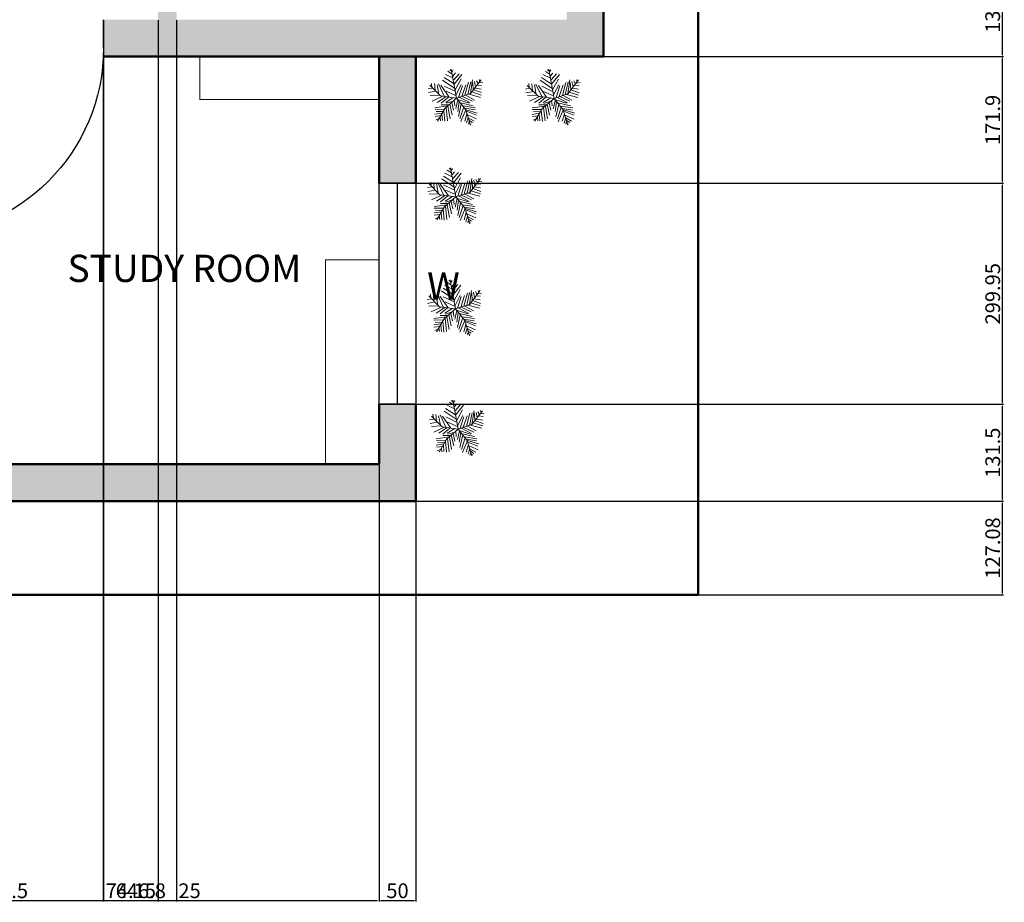
# Model space of a CAD drawing. Units: millimetres. Extents: x 1898 to 8115, y 727 to 4291.
# Tile 6 of 7: x 6778 to 8115, y 1079 to 2277. Entities that reach past the tile are written whole.
import ezdxf

# ---------------------------------------------------------------- set-up
doc = ezdxf.new("R2010")
doc.units = ezdxf.units.MM
for name, color, linetype, lineweight in [('A-ANNO-DIMS', 2, 'Continuous', 18), ('A-ANNO-TEXT', 7, 'Continuous', 25), ('A-AREA-IDEN', 3, 'Continuous', 25), ('A-DOOR', 3, 'Continuous', 25), ('A-FURN', 8, 'Continuous', 18), ('A-GLAZ', 4, 'Continuous', 25), ('A-WALL', 7, 'Continuous', 50), ('A-WALL-PATT', 8, 'Continuous', 13), ('L-PLNT', 112, 'Continuous', 18)]:
    doc.layers.add(name, color=color, linetype=linetype, lineweight=lineweight)
doc.styles.get("Standard").update_dxf_attribs({"font": 'arial.ttf'})
doc.dimstyles.new('ISO-25', dxfattribs={"dimtxt": 20, "dimasz": 2.5, "dimexe": 1.25, "dimexo": 0.625, "dimtad": 1, "dimtxsty": 'Standard', "dimcen": 2.5, "dimadec": 0, "dimazin": 0, "dimtfac": 1, "dimtmove": 0, "dimatfit": 3, "dimfxl": 1, "dimarcsym": 0})

# ---------------------------------------------------------------- blocks, each defined once
blk = doc.blocks.new('*U43')
for p, q in [((0, 0), (0, -6)), ((40, 0), (40, -6))]:
    blk.add_line(p, q)
blk.add_lwpolyline([(0, 0), (0, 40), (1.75, 40), (1.75, 0)], close=True)
blk.add_arc((0, 0), 40, 0, 90)
blk = doc.blocks.new('*U47')
for p, q in [((-5.114, 28.097), (-24.676, 40.636)), ((-7.288, 39.707), (-21.778, 46.673)), ((-8.737, 47.138), (-17.069, 52.711)), ((-10.186, 53.64), (-13.084, 55.962)), ((0, 0), (-10.5, 57)), ((-9.099, 51.782), (-6.563, 55.962)), ((-7.65, 43.423), (-2.578, 49.46)), ((-5.839, 35.992), (4.667, 48.067)), ((-5.114, 27.632), (10.463, 46.673)), ((-47.498, 19.737), (-55.83, 18.344)), ((-31.5, 4.5), (-52.5, 25.5)), ((-48.585, 21.131), (-49.309, 29.026)), ((-43.513, 28.561), (-42.427, 15.558)), ((-38.442, 26.239), (-34.819, 7.663)), ((-35.544, 28.097), (-24.314, 3.947)), ((-14.533, 2.09), (-30.834, 25.31)), ((-3.665, 19.273), (-27.574, 35.527)), ((-24.314, 23.917), (-2.941, 13.7)), ((-2.941, 16.486), (8.652, 37.85)), ((-1.129, 6.734), (9.014, 26.704)), ((3.942, 1.625), (11.187, 24.381)), ((10.101, 3.483), (17.708, 26.239)), ((16.259, 5.805), (23.142, 31.348)), ((22.055, 7.198), (27.489, 32.277)), ((27, 9), (48, 36)), ((27.127, 9.056), (31.112, 35.992)), ((31.836, 30.883), (32.561, 16.486)), ((35.096, 32.741), (37.27, 22.524)), ((36.183, 19.737), (48.137, 17.88)), ((38.719, 34.134), (41.979, 28.561)), ((40.53, 25.775), (48.862, 24.846)), ((43.791, 29.954), (51.036, 30.883)), ((44.153, 36.456), (45.239, 32.741)), ((-40.615, 13.7), (-55.105, 10.913)), ((-33.37, 6.269), (-52.207, 5.34)), ((-28.299, 3.483), (-47.86, -5.805)), ((-21.416, 3.018), (-38.079, -8.128)), ((0, 0), (-31.5, 4.5)), ((-15.982, 2.09), (-30.11, -9.521)), ((0, 0), (-22.5, -19.5)), ((-6.563, 1.161), (-21.416, -8.128)), ((-20.691, 13.7), (-1.129, 4.876)), ((0, 0), (27, 9)), ((0, 0), (18, -22.5)), ((6.478, 1.625), (26.04, -8.592)), ((11.187, 3.483), (30.749, -5.805)), ((18.07, 5.805), (35.096, -3.483)), ((24.229, 7.663), (46.688, 1.625)), ((29.662, 12.307), (48.137, 6.269)), ((33.285, 16.486), (48.862, 10.913)), ((-17.431, -15.094), (-42.789, -18.809)), ((-15.257, -12.772), (-30.11, -12.772)), ((-20.691, -18.345), (-17.793, -44.352)), ((-6.563, -5.805), (-19.967, -9.985)), ((-17.069, -15.094), (-12.721, -40.172)), ((-13.446, -11.378), (-8.737, -32.741)), ((-9.461, -8.592), (-6.201, -23.453)), ((-4.752, -3.483), (-3.665, -14.629)), ((2.493, -3.019), (-1.491, -20.202)), ((1.769, -2.555), (24.229, -9.521)), ((5.029, -6.27), (2.131, -25.775)), ((9.014, -11.378), (3.58, -35.992)), ((14.085, -16.951), (6.478, -40.172)), ((7.565, -9.056), (32.198, -14.629)), ((12.274, -15.094), (36.907, -18.809)), ((-28.299, -29.026), (-42.789, -31.348)), ((-24.314, -21.596), (-42.427, -22.06)), ((-30.834, -34.135), (-42.427, -35.528)), ((-26.849, -26.24), (-40.253, -25.775)), ((-22.5, -19.5), (-37.5, -45)), ((-32.646, -36.921), (-31.921, -44.352)), ((-29.023, -30.884), (-27.936, -43.887)), ((-25.038, -23.918), (-22.865, -45.281)), ((18.07, -22.524), (8.289, -45.745)), ((20.244, -30.419), (15.897, -44.816)), ((16.259, -19.738), (36.183, -22.989)), ((18, -22.5), (27, -52.5)), ((18.433, -22.524), (40.53, -29.026)), ((19.157, -25.311), (38.719, -33.206)), ((22.78, -37.85), (19.519, -48.532)), ((21.331, -32.741), (39.081, -40.636)), ((22.78, -38.314), (34.372, -44.816)), ((-34.457, -39.708), (-40.978, -42.494)), ((24.591, -45.745), (23.142, -50.854)), ((24.591, -43.423), (30.749, -47.603)), ((26.764, -49.925), (28.213, -50.854))]:
    blk.add_line(p, q)
blk = doc.blocks.new('*D62')
at = {"layer": 'A-ANNO-DIMS', "color": 0, "lineweight": -2, "transparency": 16777216}
for p, q in [((7316.4, 1623.6), (8113.5, 1623.6)), ((8112.2, 1499), (8112.2, 1621.1)), ((7699.4, 1496.5), (8113.5, 1496.5))]:
    blk.add_line(p, q, dxfattribs=at)
at = {"layer": 'A-ANNO-DIMS', "color": 0, "transparency": 16777216}
for points in [[(8111.8, 1621.1), (8112.7, 1621.1), (8112.2, 1623.6)], [(8111.8, 1499), (8112.7, 1499), (8112.2, 1496.5)]]:
    blk.add_solid(points, dxfattribs=at)
at = {"layer": 'Defpoints', "color": 0, "transparency": 16777216}
for p in [(7315.8, 1623.6), (8112.2, 1623.6), (7698.8, 1496.5)]:
    blk.add_point(p, dxfattribs=at)
at = {"layer": 'A-ANNO-DIMS', "color": 0, "transparency": 16777216, "insert": (8101.4, 1560.1), "char_height": 20, "attachment_point": 5, "rotation": 90}
blk.add_mtext('127.08', dxfattribs=at)
blk = doc.blocks.new('*D77')
at = {"layer": 'A-ANNO-DIMS', "color": 0, "lineweight": -2, "transparency": 16777216}
for p, q in [((6618.9, 1673), (6618.9, 1080.3)), ((7265.8, 1673), (7265.8, 1080.3)), ((6621.4, 1081.6), (7263.3, 1081.6))]:
    blk.add_line(p, q, dxfattribs=at)
at = {"layer": 'A-ANNO-DIMS', "color": 0, "transparency": 16777216}
for points in [[(6621.4, 1082), (6621.4, 1081.2), (6618.9, 1081.6)], [(7263.3, 1082), (7263.3, 1081.2), (7265.8, 1081.6)]]:
    blk.add_solid(points, dxfattribs=at)
at = {"layer": 'Defpoints', "color": 0, "transparency": 16777216}
for p in [(6618.9, 1673.6), (7265.8, 1673.6), (7265.8, 1081.6)]:
    blk.add_point(p, dxfattribs=at)
at = {"layer": 'A-ANNO-DIMS', "color": 0, "transparency": 16777216, "insert": (6942.3, 1092.4), "char_height": 20, "attachment_point": 5}
blk.add_mtext('646.8', dxfattribs=at)
blk = doc.blocks.new('*D78')
at = {"layer": 'A-ANNO-DIMS', "color": 0, "lineweight": -2, "transparency": 16777216}
for p, q in [((7265.8, 1673), (7265.8, 1080.3)), ((7315.8, 1623), (7315.8, 1080.3)), ((7268.3, 1081.6), (7313.3, 1081.6))]:
    blk.add_line(p, q, dxfattribs=at)
at = {"layer": 'A-ANNO-DIMS', "color": 0, "transparency": 16777216}
for points in [[(7268.3, 1082), (7268.3, 1081.2), (7265.8, 1081.6)], [(7313.3, 1082), (7313.3, 1081.2), (7315.8, 1081.6)]]:
    blk.add_solid(points, dxfattribs=at)
at = {"layer": 'Defpoints', "color": 0, "transparency": 16777216}
for p in [(7265.8, 1673.6), (7315.8, 1623.6), (7315.8, 1081.6)]:
    blk.add_point(p, dxfattribs=at)
at = {"layer": 'A-ANNO-DIMS', "color": 0, "transparency": 16777216, "insert": (7290.8, 1092.4), "char_height": 20, "attachment_point": 5}
blk.add_mtext('50', dxfattribs=at)
blk = doc.blocks.new('*D91')
at = {"layer": 'A-ANNO-DIMS', "color": 0, "lineweight": -2, "transparency": 16777216}
for p, q in [((7316.4, 1755.1), (8113.5, 1755.1)), ((8112.2, 1626.1), (8112.2, 1752.6)), ((7316.4, 1623.6), (8113.5, 1623.6))]:
    blk.add_line(p, q, dxfattribs=at)
at = {"layer": 'A-ANNO-DIMS', "color": 0, "transparency": 16777216}
for points in [[(8111.8, 1752.6), (8112.7, 1752.6), (8112.2, 1755.1)], [(8111.8, 1626.1), (8112.7, 1626.1), (8112.2, 1623.6)]]:
    blk.add_solid(points, dxfattribs=at)
at = {"layer": 'Defpoints', "color": 0, "transparency": 16777216}
for p in [(7315.8, 1755.1), (8112.2, 1755.1), (7315.8, 1623.6)]:
    blk.add_point(p, dxfattribs=at)
at = {"layer": 'A-ANNO-DIMS', "color": 0, "transparency": 16777216, "insert": (8101.4, 1689.4), "char_height": 20, "attachment_point": 5, "rotation": 90}
blk.add_mtext('131.5', dxfattribs=at)
blk = doc.blocks.new('*D92')
at = {"layer": 'A-ANNO-DIMS', "color": 0, "lineweight": -2, "transparency": 16777216}
for p, q in [((7316.4, 2055.1), (8113.5, 2055.1)), ((8112.2, 1757.6), (8112.2, 2052.6)), ((7316.4, 1755.1), (8113.5, 1755.1))]:
    blk.add_line(p, q, dxfattribs=at)
at = {"layer": 'A-ANNO-DIMS', "color": 0, "transparency": 16777216}
for points in [[(8111.8, 2052.6), (8112.7, 2052.6), (8112.2, 2055.1)], [(8111.8, 1757.6), (8112.7, 1757.6), (8112.2, 1755.1)]]:
    blk.add_solid(points, dxfattribs=at)
at = {"layer": 'Defpoints', "color": 0, "transparency": 16777216}
for p in [(7315.8, 2055.1), (8112.2, 2055.1), (7315.8, 1755.1)]:
    blk.add_point(p, dxfattribs=at)
at = {"layer": 'A-ANNO-DIMS', "color": 0, "transparency": 16777216, "insert": (8101.4, 1905.1), "char_height": 20, "attachment_point": 5, "rotation": 90}
blk.add_mtext('299.95', dxfattribs=at)
blk = doc.blocks.new('*D93')
at = {"layer": 'A-ANNO-DIMS', "color": 0, "lineweight": -2, "transparency": 16777216}
for p, q in [((7316.4, 2227), (8113.5, 2227)), ((8112.2, 2057.6), (8112.2, 2224.5)), ((7316.4, 2055.1), (8113.5, 2055.1))]:
    blk.add_line(p, q, dxfattribs=at)
at = {"layer": 'A-ANNO-DIMS', "color": 0, "transparency": 16777216}
for points in [[(8111.8, 2224.5), (8112.7, 2224.5), (8112.2, 2227)], [(8111.8, 2057.6), (8112.7, 2057.6), (8112.2, 2055.1)]]:
    blk.add_solid(points, dxfattribs=at)
at = {"layer": 'Defpoints', "color": 0, "transparency": 16777216}
for p in [(7315.8, 2227), (8112.2, 2227), (7315.8, 2055.1)]:
    blk.add_point(p, dxfattribs=at)
at = {"layer": 'A-ANNO-DIMS', "color": 0, "transparency": 16777216, "insert": (8101.4, 2141), "char_height": 20, "attachment_point": 5, "rotation": 90}
blk.add_mtext('171.9', dxfattribs=at)
blk = doc.blocks.new('*D94')
at = {"layer": 'A-ANNO-DIMS', "color": 0, "lineweight": -2, "transparency": 16777216}
for p, q in [((7570.8, 2359.5), (8113.5, 2359.5)), ((8112.2, 2229.5), (8112.2, 2357)), ((7570.8, 2227), (8113.5, 2227))]:
    blk.add_line(p, q, dxfattribs=at)
at = {"layer": 'A-ANNO-DIMS', "color": 0, "transparency": 16777216}
for points in [[(8111.8, 2357), (8112.7, 2357), (8112.2, 2359.5)], [(8111.8, 2229.5), (8112.7, 2229.5), (8112.2, 2227)]]:
    blk.add_solid(points, dxfattribs=at)
at = {"layer": 'Defpoints', "color": 0, "transparency": 16777216}
for p in [(7570.2, 2359.5), (8112.2, 2359.5), (7570.2, 2227)]:
    blk.add_point(p, dxfattribs=at)
at = {"layer": 'A-ANNO-DIMS', "color": 0, "transparency": 16777216, "insert": (8101.4, 2293.2), "char_height": 20, "attachment_point": 5, "rotation": 90}
blk.add_mtext('132.5', dxfattribs=at)
blk = doc.blocks.new('*D107')
at = {"layer": 'A-ANNO-DIMS', "color": 0, "lineweight": -2, "transparency": 16777216}
for p, q in [((6618.9, 2226.3), (6618.9, 1080.3)), ((6891.4, 2226.3), (6891.4, 1080.3)), ((6621.4, 1081.6), (6888.9, 1081.6))]:
    blk.add_line(p, q, dxfattribs=at)
at = {"layer": 'A-ANNO-DIMS', "color": 0, "transparency": 16777216}
for points in [[(6621.4, 1082), (6621.4, 1081.2), (6618.9, 1081.6)], [(6888.9, 1082), (6888.9, 1081.2), (6891.4, 1081.6)]]:
    blk.add_solid(points, dxfattribs=at)
at = {"layer": 'Defpoints', "color": 0, "transparency": 16777216}
for p in [(6618.9, 2227), (6891.4, 2227), (6891.4, 1081.6)]:
    blk.add_point(p, dxfattribs=at)
at = {"layer": 'A-ANNO-DIMS', "color": 0, "transparency": 16777216, "insert": (6755.2, 1092.4), "char_height": 20, "attachment_point": 5}
blk.add_mtext('272.5', dxfattribs=at)
blk = doc.blocks.new('*D108')
at = {"layer": 'A-ANNO-DIMS', "color": 0, "lineweight": -2, "transparency": 16777216}
for p, q in [((6891.7, 2276.3), (6891.7, 1080.3)), ((6965.8, 2276.3), (6965.8, 1080.3)), ((6894.2, 1081.6), (6963.3, 1081.6))]:
    blk.add_line(p, q, dxfattribs=at)
at = {"layer": 'A-ANNO-DIMS', "color": 0, "transparency": 16777216}
for points in [[(6894.2, 1082), (6894.2, 1081.2), (6891.7, 1081.6)], [(6963.3, 1082), (6963.3, 1081.2), (6965.8, 1081.6)]]:
    blk.add_solid(points, dxfattribs=at)
at = {"layer": 'Defpoints', "color": 0, "transparency": 16777216}
for p in [(6891.7, 2277), (6965.8, 2277), (6965.8, 1081.6)]:
    blk.add_point(p, dxfattribs=at)
at = {"layer": 'A-ANNO-DIMS', "color": 0, "transparency": 16777216, "insert": (6928.8, 1092.4), "char_height": 20, "attachment_point": 5}
blk.add_mtext('74.15', dxfattribs=at)
blk = doc.blocks.new('*D109')
at = {"layer": 'A-ANNO-DIMS', "color": 0, "lineweight": -2, "transparency": 16777216}
for p, q in [((6965.8, 2276.3), (6965.8, 1080.3)), ((6990.8, 2276.3), (6990.8, 1080.3)), ((6968.3, 1081.6), (6988.3, 1081.6)), ((6990.8, 1081.6), (7023.7, 1081.6))]:
    blk.add_line(p, q, dxfattribs=at)
at = {"layer": 'A-ANNO-DIMS', "color": 0, "transparency": 16777216}
for points in [[(6968.3, 1082), (6968.3, 1081.2), (6965.8, 1081.6)], [(6988.3, 1082), (6988.3, 1081.2), (6990.8, 1081.6)]]:
    blk.add_solid(points, dxfattribs=at)
at = {"layer": 'Defpoints', "color": 0, "transparency": 16777216}
for p in [(6965.8, 2277), (6990.8, 2277), (6990.8, 1081.6)]:
    blk.add_point(p, dxfattribs=at)
at = {"layer": 'A-ANNO-DIMS', "color": 0, "transparency": 16777216, "insert": (7008.5, 1092.4), "char_height": 20, "attachment_point": 5}
blk.add_mtext('25', dxfattribs=at)

msp = doc.modelspace()

# ---------------------------------------------------------------- hatches: boundary and pattern name
at = {"layer": 'A-WALL-PATT'}
h = msp.add_hatch(color=256, dxfattribs=at)
h.dxf.hatch_style = 1
h.paths.add_polyline_path([(6201.726, 3440.661), (5461.585, 3440.661), (5461.585, 3265.221), (5511.585, 3265.221), (5511.585, 3390.661), (6176.726, 3390.661), (6176.726, 2856.284), (6201.726, 2856.284)])
h.paths.add_polyline_path([(6784.895, 3318.017), (6201.726, 3318.017), (6201.726, 3268.017), (6784.895, 3268.017)])
h.paths.add_polyline_path([(7570.217, 3440.661), (6784.895, 3440.661), (6784.895, 3057.009), (6809.895, 3057.009), (6809.895, 3390.661), (7520.217, 3390.661), (7520.217, 3300.311), (7570.217, 3300.311)])
h.paths.add_polyline_path([(7570.217, 3000.359), (7520.217, 3000.359), (7520.217, 2758.681), (7570.217, 2758.681)])
h.paths.add_polyline_path([(7520.217, 2856.284), (7194.283, 2856.284), (6784.895, 2856.284), (6784.895, 2831.284), (7520.217, 2831.284)])
h.paths.add_polyline_path([(6809.895, 2878.069), (6784.895, 2878.069), (6784.895, 2856.284), (6809.895, 2856.284)])
h.paths.add_polyline_path([(6201.726, 2856.284), (6176.726, 2856.284), (6161.551, 2856.284), (6161.551, 2831.284), (6201.726, 2831.284)])
h.paths.add_polyline_path([(5905.861, 2856.284), (5511.585, 2856.284), (5511.585, 2831.284), (5905.861, 2831.284)])
h.paths.add_polyline_path([(5511.585, 2965.269), (5461.585, 2965.269), (5461.585, 2698.678), (5511.585, 2698.678)])
h.paths.add_polyline_path([(5511.585, 2398.725), (5461.585, 2398.725), (5461.585, 2088.028), (5511.585, 2088.028)])
h.paths.add_polyline_path([(5989.6, 2238.621), (5989.6, 2276.975), (5511.585, 2276.975), (5511.585, 2226.975), (5989.865, 2226.975, -0.01139164)])
h.paths.add_polyline_path([(6636.013, 2276.975), (6245.29, 2276.975), (6245.29, 2238.621), (6245.29, 2226.975), (6636.013, 2226.975), (6636.013, 2238.621)])
h.paths.add_polyline_path([(7570.217, 2359.481), (7520.217, 2359.481), (7520.217, 2326.802), (7520.217, 2276.975), (6891.704, 2276.975), (6891.704, 2238.621, -0.01139164), (6891.439, 2226.975), (7570.217, 2226.975)])
h.paths.add_polyline_path([(7145.586, 2531.644), (6989.313, 2531.644), (6989.313, 2538.488), (7145.735, 2538.488), (7145.735, 2531.644), (7145.586, 2531.644, -0.39860379), (6990.849, 2382.073), (6990.849, 2276.975), (6965.849, 2276.975), (6965.849, 2382.065), (6989.313, 2382.065, 0.40145271)])
h.paths.add_polyline_path([(6990.849, 2596.561), (6989.313, 2596.561), (6965.849, 2596.561), (6965.849, 2538.488), (6990.849, 2538.488)])
h.paths.add_polyline_path([(6990.849, 2831.284), (6965.849, 2831.284), (6965.849, 2752.984), (6990.849, 2752.984)])
h.paths.add_polyline_path([(7570.217, 2638.517), (7520.217, 2638.517), (7520.217, 2625.002), (7520.217, 2479.644), (7570.217, 2479.644)])
h.paths.add_polyline_path([(7520.217, 2579.13), (6990.849, 2579.13), (6990.849, 2554.13), (7520.217, 2554.13)])
h = msp.add_hatch(color=256, dxfattribs=at)
h.dxf.hatch_style = 1
h.paths.add_polyline_path([(6362.741, 1673.621), (6361.204, 1673.621), (5511.585, 1673.621), (5511.585, 1788.076), (5461.585, 1788.076), (5461.585, 1623.621), (6362.741, 1623.621)])
h.paths.add_polyline_path([(7315.762, 1755.132), (7265.762, 1755.132), (7265.762, 1673.621), (6520.151, 1673.621), (6520.151, 1623.621), (7315.762, 1623.621)])
h.paths.add_polyline_path([(7315.762, 2226.975), (7265.762, 2226.975), (7265.762, 2168.705), (7265.762, 2055.084), (7315.762, 2055.084)])
h.paths.add_polyline_path([(6618.931, 1855.35), (6618.931, 2226.975), (6593.931, 2226.975), (6593.931, 1673.621), (6618.931, 1673.621)])
h.paths.add_polyline_path([(6305.461, 2043.361), (6280.461, 2043.361), (6280.461, 1673.621), (6305.461, 1673.621)])
h.paths.add_polyline_path([(6305.461, 2226.975), (6280.461, 2226.975), (6280.461, 2209.076), (6305.461, 2209.076)])

# ---------------------------------------------------------------- linework, layer by layer
at = {"layer": 'A-FURN'}
msp.add_lwpolyline([(7265.762, 2226.975), (7022.614, 2226.975), (7022.614, 2168.705), (7265.762, 2168.705)], close=True, dxfattribs=at)
msp.add_lwpolyline([(7265.762, 1755.132), (7265.762, 1673.621), (7192.879, 1673.621), (7192.879, 1950.944), (7265.762, 1950.944)], dxfattribs=at)
at = {"layer": 'A-GLAZ'}
msp.add_line((7290.762, 1755.132), (7290.762, 2055.084), dxfattribs=at)
for points in [[(7315.762, 2055.084), (7265.762, 2055.084)], [(7265.762, 1755.132), (7315.762, 1755.132)]]:
    msp.add_lwpolyline(points, dxfattribs=at)
msp.add_lwpolyline([(7315.762, 1755.132), (7265.762, 1755.132), (7265.762, 2055.084), (7315.762, 2055.084)], close=True, dxfattribs=at)
at = {"layer": 'A-WALL'}
for p, q in [((7570.217, 2359.481), (7570.217, 2226.975)), ((6891.439, 2226.975), (7570.217, 2226.975)), ((7265.762, 2226.975), (7265.762, 2055.084)), ((7315.762, 2226.975), (7315.762, 2055.084)), ((7265.762, 1755.132), (7265.762, 1673.621)), ((7315.762, 1755.132), (7315.762, 1623.621)), ((5511.585, 1673.621), (7265.762, 1673.621)), ((6520.151, 1623.621), (7315.762, 1623.621))]:
    msp.add_line(p, q, dxfattribs=at)
msp.add_lwpolyline([(5348.551, 3559.737), (7698.767, 3559.737), (7698.767, 1496.544), (5348.551, 1496.544)], close=True, dxfattribs=at)

# ---------------------------------------------------------------- block references
at = {"layer": 'A-DOOR', "xscale": -6.392265120440044, "yscale": 6.392265120440044, "zscale": 6.392265120440044, "rotation": 180}
msp.add_blockref('*U43', (6636.013, 2238.621), dxfattribs=at)
at = {"layer": 'L-PLNT', "xscale": 0.6924237731587986, "yscale": 0.6924237731587986, "zscale": 0.6924237731587986}
for p in [(7371.099, 2170.415), (7503.352, 2170.233), (7370.154, 2036.389), (7369.693, 1884.43), (7373.119, 1721.368)]:
    msp.add_blockref('*U47', p, dxfattribs=at)

# ---------------------------------------------------------------- texts
at = {"layer": 'A-ANNO-TEXT', "insert": (7331.035, 1934.113), "char_height": 36.981, "attachment_point": 1}
msp.add_mtext_dynamic_manual_height_columns('W', width=5503.90807, gutter_width=184.907, heights=[0], dxfattribs=at)
at = {"layer": 'A-AREA-IDEN', "insert": (6842.853, 1958.021), "char_height": 36.9814, "attachment_point": 1}
msp.add_mtext_dynamic_manual_height_columns('STUDY ROOM', width=5503.90807, gutter_width=184.907, heights=[0], dxfattribs=at)

# ---------------------------------------------------------------- dimensions: what is measured, and where the dimension line sits
at = {"layer": 'A-ANNO-DIMS'}
for base, p1, p2, override, picture, middle in [((8112.244, 2359.481), (7570.217, 2226.975), (7570.217, 2359.481), {"dimdec": 1, "dimlfac": 1, "dimrnd": 0, "dimzin": 0, "dimdsep": 46, "dimlunit": 2}, '*D94', (8101.401, 2293.228)), ((8112.244, 2226.975), (7315.762, 2055.084), (7315.762, 2226.975), {"dimdec": 1, "dimlfac": 1, "dimrnd": 0, "dimzin": 0, "dimdsep": 46, "dimlunit": 2}, '*D93', (8101.408, 2141.029)), ((8112.244, 2055.084), (7315.762, 1755.132), (7315.762, 2055.084), {"dimdec": 2, "dimlfac": 1, "dimrnd": 0, "dimzin": 0, "dimdsep": 46, "dimlunit": 2}, '*D92', (8101.408, 1905.108)), ((8112.244, 1755.132), (7315.762, 1623.621), (7315.762, 1755.132), {"dimdec": 1, "dimlfac": 1, "dimrnd": 0, "dimzin": 0, "dimdsep": 46, "dimlunit": 2}, '*D91', (8101.401, 1689.376)), ((8112.244, 1623.621), (7698.767, 1496.544), (7315.762, 1623.621), {"dimdec": 2, "dimlfac": 1, "dimrnd": 0, "dimzin": 0, "dimdsep": 46, "dimlunit": 2}, '*D62', (8101.408, 1560.082))]:
    dim = msp.add_linear_dim(base=base, p1=p1, p2=p2, angle=90, dimstyle='ISO-25', override=override, dxfattribs=at)
    dim.commit()
    dim.dimension.update_dxf_attribs({"geometry": picture, "text_midpoint": middle})
for base, p1, p2, override, picture, middle in [((6965.8494, 1081.5935), (6891.704, 2276.9748), (6965.8494, 2276.9748), {"dimdec": 2, "dimlfac": 1, "dimrnd": 0, "dimzin": 0, "dimdsep": 46, "dimlunit": 2}, '*D108', (6928.7767, 1092.43)), ((6990.849, 1081.594), (6965.849, 2276.975), (6990.849, 2276.975), {"dimdec": 0, "dimlfac": 1, "dimrnd": 0, "dimzin": 0, "dimdsep": 46, "dimlunit": 2}, '*D109', (7008.545, 1092.43)), ((6891.439, 1081.594), (6618.931, 2226.975), (6891.439, 2226.975), {"dimdec": 1, "dimlfac": 1, "dimrnd": 0, "dimzin": 0, "dimdsep": 46, "dimlunit": 2}, '*D107', (6755.185, 1092.43)), ((7265.762, 1081.594), (6618.931, 1673.621), (7265.762, 1673.621), {"dimdec": 1, "dimlfac": 1, "dimrnd": 0, "dimzin": 0, "dimdsep": 46, "dimlunit": 2}, '*D77', (6942.347, 1092.43)), ((7315.762, 1081.594), (7265.762, 1673.621), (7315.762, 1623.621), {"dimdec": 0, "dimlfac": 1, "dimrnd": 0, "dimzin": 0, "dimdsep": 46, "dimlunit": 2}, '*D78', (7290.762, 1092.43))]:
    dim = msp.add_linear_dim(base=base, p1=p1, p2=p2, dimstyle='ISO-25', override=override, dxfattribs=at)
    dim.commit()
    dim.dimension.update_dxf_attribs({"geometry": picture, "text_midpoint": middle})

doc.saveas('drawing.dxf')
